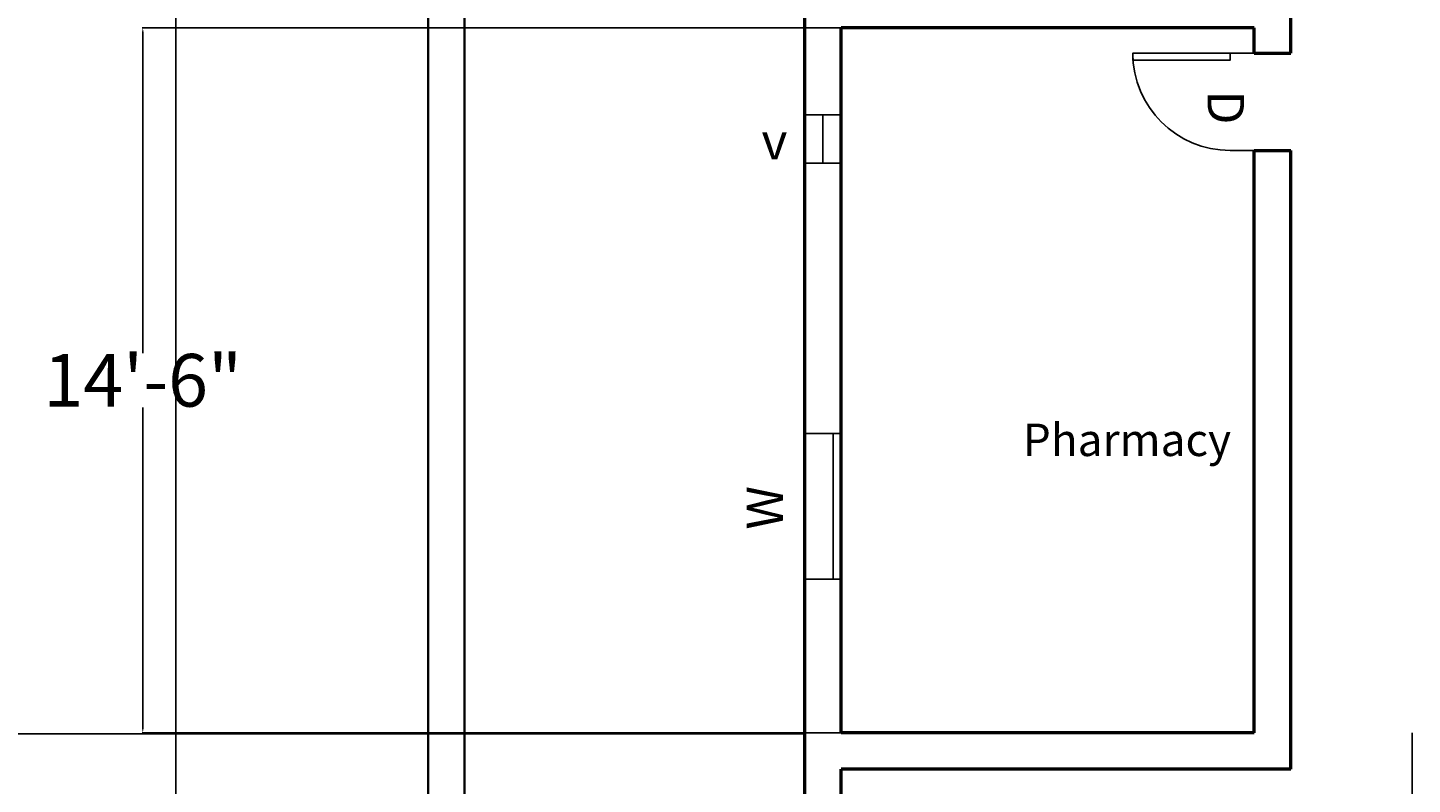
# Model space of a CAD drawing. Units: inches. Extents: x -364 to 705, y -52 to 1250.
# Tile 3 of 34: x -163 to 179, y 136 to 323. Entities that reach past the tile are written whole.
import ezdxf

# ---------------------------------------------------------------- set-up
doc = ezdxf.new("R2010")
doc.units = ezdxf.units.IN
doc.header["$MEASUREMENT"] = 0
for name, color, linetype, lineweight in [('A-ANNO-DIMS', 4, 'Continuous', 18), ('A-ANNO-IDEN', 1, 'Continuous', 18), ('A-AREA-IDEN', 3, 'Continuous', 18), ('A-DOOR', 1, 'Continuous', 25), ('A-FLOR-RAMP', 7, 'Continuous', 25), ('A-GLAZ', 4, 'Continuous', 25), ('A-WALL', 41, 'Continuous', 50), ('C-WALL', 41, 'Continuous', 35)]:
    doc.layers.add(name, color=color, linetype=linetype, lineweight=lineweight)
doc.styles.get("Standard").update_dxf_attribs({"font": 'arial.ttf'})
doc.dimstyles.get("Standard").update_dxf_attribs({"dimtxt": 1, "dimasz": 1, "dimexe": 0.18, "dimexo": 0.0625, "dimgap": 0.09, "dimtad": 0, "dimtih": 1, "dimtoh": 1, "dimdec": 0, "dimzin": 0, "dimdsep": 46, "dimlunit": 3, "dimtxsty": 'Standard', "dimcen": 0.09, "dimadec": 0, "dimazin": 0, "dimtfac": 1, "dimtdec": 0, "dimtofl": 0, "dimtmove": 0, "dimatfit": 3, "dimfxl": 1, "dimtolj": 1, "dimtzin": 0, "dimarcsym": 0})

# ---------------------------------------------------------------- blocks, each defined once
blk = doc.blocks.new('*U16')
for p, q in [((-24, 0), (-24, 6)), ((0, 0), (0, 6))]:
    blk.add_line(p, q)
blk.add_lwpolyline([(0, 0), (0, -24), (-1.75, -24), (-1.75, 0)], close=True)
blk.add_arc((0, 0), 24, 180, 270)
blk = doc.blocks.new('*D19')
at = {"layer": 'A-ANNO-DIMS', "color": 0, "lineweight": -2, "transparency": 16777216}
for p, q in [((28.52, 986.11), (-248.33, 986.11)), ((-248.15, 985.11), (-248.15, 574.22)), ((-248.15, 149.87), (-248.15, 560.77)), ((28.52, 148.87), (-248.33, 148.87))]:
    blk.add_line(p, q, dxfattribs=at)
at = {"layer": 'A-ANNO-DIMS', "color": 0, "transparency": 16777216}
for points in [[(-248.32, 985.11), (-247.99, 985.11), (-248.15, 986.11)], [(-248.32, 149.87), (-247.99, 149.87), (-248.15, 148.87)]]:
    blk.add_solid(points, dxfattribs=at)
at = {"layer": 'Defpoints', "color": 0, "transparency": 16777216}
for p in [(28.58, 986.11), (-248.15, 148.87), (28.58, 148.87)]:
    blk.add_point(p, dxfattribs=at)
at = {"layer": 'A-ANNO-DIMS', "color": 0, "transparency": 16777216, "insert": (-248.15, 567.49), "char_height": 1, "attachment_point": 5}
blk.add_mtext('\\A1;{\\H13x;69\'-9"}', dxfattribs=at)
blk = doc.blocks.new('*D28')
at = {"layer": 'A-ANNO-DIMS', "color": 0, "lineweight": -2, "transparency": 16777216}
for p, q in [((37.52, 323.11), (-135.02, 323.11)), ((-134.84, 322.11), (-134.84, 242.84)), ((-134.84, 150.11), (-134.84, 229.39)), ((37.52, 149.11), (-135.02, 149.11))]:
    blk.add_line(p, q, dxfattribs=at)
at = {"layer": 'A-ANNO-DIMS', "color": 0, "transparency": 16777216}
for points in [[(-135.01, 322.11), (-134.67, 322.11), (-134.84, 323.11)], [(-135.01, 150.11), (-134.67, 150.11), (-134.84, 149.11)]]:
    blk.add_solid(points, dxfattribs=at)
at = {"layer": 'Defpoints', "color": 0, "transparency": 16777216}
for p in [(-134.84, 323.11), (37.58, 323.11), (37.58, 149.11)]:
    blk.add_point(p, dxfattribs=at)
at = {"layer": 'A-ANNO-DIMS', "color": 0, "transparency": 16777216, "insert": (-134.84, 236.11), "char_height": 1, "attachment_point": 5}
blk.add_mtext('\\A1;{\\H13x;14\'-6"}', dxfattribs=at)
blk = doc.blocks.new('VENT-12')
blk.add_line((4.51, 0), (4.51, 12))
blk.add_lwpolyline([(9, 0), (9, 12), (0, 12), (0, 0)], close=True)
blk = doc.blocks.new('*D76')
at = {"layer": 'A-ANNO-DIMS', "color": 0, "lineweight": -2, "transparency": 16777216}
for p, q in [((28.52, 986.11), (-126.85, 986.11)), ((-126.67, 985.11), (-126.67, 499.22)), ((-126.67, 12.11), (-126.67, 498.01)), ((28.52, 11.11), (-126.85, 11.11))]:
    blk.add_line(p, q, dxfattribs=at)
at = {"layer": 'A-ANNO-DIMS', "color": 0, "transparency": 16777216}
for points in [[(-126.84, 985.11), (-126.5, 985.11), (-126.67, 986.11)], [(-126.84, 12.11), (-126.5, 12.11), (-126.67, 11.11)]]:
    blk.add_solid(points, dxfattribs=at)
at = {"layer": 'Defpoints', "color": 0, "transparency": 16777216}
for p in [(-126.67, 986.11), (28.58, 986.11), (28.58, 11.11)]:
    blk.add_point(p, dxfattribs=at)
at = {"layer": 'A-ANNO-DIMS', "color": 0, "transparency": 16777216, "insert": (-126.67, 498.61), "char_height": 1, "attachment_point": 5}
blk.add_mtext('\\A1;81\'-3"', dxfattribs=at)

msp = doc.modelspace()

# ---------------------------------------------------------------- linework, layer by layer
at = {"layer": 'A-FLOR-RAMP'}
msp.add_line((178.58, 11.11), (178.58, 149.11), dxfattribs=at)
at = {"layer": 'A-GLAZ'}
for p, q in [((35.58, 223.01), (35.58, 187.01)), ((37.58, 223.01), (37.58, 187.01))]:
    msp.add_line(p, q, dxfattribs=at)
msp.add_lwpolyline([(37.58, 223.01), (37.58, 187.01), (28.58, 187.01), (28.58, 223.01)], close=True, dxfattribs=at)
at = {"layer": 'A-WALL'}
for p, q in [((28.58, 11.11), (28.58, 986.11)), ((148.58, 316.83), (148.58, 422.97)), ((139.58, 323.11), (37.58, 323.11)), ((37.58, 149.11), (37.58, 323.11)), ((139.58, 316.83), (139.58, 323.11)), ((139.58, 316.83), (139.58, 321.83)), ((139.58, 316.83), (148.58, 316.83)), ((139.58, 149.11), (139.58, 292.83)), ((139.58, 292.83), (148.58, 292.83)), ((148.58, 140.11), (148.58, 292.83)), ((139.58, 149.11), (37.58, 149.11)), ((37.58, 20.11), (37.58, 140.11)), ((148.58, 140.11), (37.58, 140.11))]:
    msp.add_line(p, q, dxfattribs=at)
at = {"layer": 'C-WALL'}
for p, q in [((-64.42, 11.11), (-64.42, 1079.11)), ((-55.42, 11.11), (-55.42, 1070.11))]:
    msp.add_line(p, q, dxfattribs=at)

# ---------------------------------------------------------------- block references
at = {"layer": 'A-DOOR', "xscale": -1, "rotation": 270.0000000000011}
msp.add_blockref('*U16', (133.58, 316.83), dxfattribs=at)
at = {"layer": 'A-GLAZ'}
msp.add_blockref('VENT-12', (28.58, 289.65), dxfattribs=at)

# ---------------------------------------------------------------- texts
at = {"layer": 'A-ANNO-IDEN', "char_height": 9, "attachment_point": 1}
for s, width, insert, rotation in [('D', 16.916, (137.04, 307.67), 270), ('W', 31.4151, (14.21, 199.25), 90)]:
    msp.add_mtext_dynamic_manual_height_columns(s, width=width, gutter_width=1, heights=[0], dxfattribs=dict(at, insert=insert, rotation=rotation))
at = {"layer": 'A-ANNO-IDEN', "insert": (17.91, 299.61), "char_height": 9, "attachment_point": 1}
msp.add_mtext_dynamic_manual_height_columns('v', width=10.6887, gutter_width=1, heights=[0], dxfattribs=at)
at = {"layer": 'A-AREA-IDEN', "insert": (82.42, 225.41), "char_height": 0.2, "attachment_point": 1}
msp.add_mtext_dynamic_manual_height_columns('{\\H40x;Pharmacy}', width=50.1257, gutter_width=1, heights=[0], dxfattribs=at)

# ---------------------------------------------------------------- dimensions: what is measured, and where the dimension line sits
at = {"layer": 'A-ANNO-DIMS'}
for base, p1, p2, picture, middle in [((-248.15, 148.87), (28.58, 986.11), (28.58, 148.87), '*D19', (-248.15, 567.49)), ((-134.84, 323.11), (37.58, 149.11), (37.58, 323.11), '*D28', (-134.84, 236.11))]:
    dim = msp.add_linear_dim(base=base, p1=p1, p2=p2, angle=90, text='{\\H13x;<>}', dimstyle='Standard', override={"dimclrd": 0, "dimclre": 0, "dimclrt": 0}, dxfattribs=at)
    dim.commit()
    dim.dimension.update_dxf_attribs({"geometry": picture, "text_midpoint": middle})
dim = msp.add_linear_dim(base=(-126.67, 986.11), p1=(28.58, 11.11), p2=(28.58, 986.11), angle=90, dimstyle='Standard', override={"dimdec": 1, "dimlfac": 1, "dimrnd": 0, "dimzin": 1, "dimdsep": 46, "dimlunit": 4, "dimfrac": 2}, dxfattribs=at)
dim.commit()
dim.dimension.update_dxf_attribs({"geometry": '*D76', "text_midpoint": (-126.67, 498.61)})

doc.saveas('drawing.dxf')
